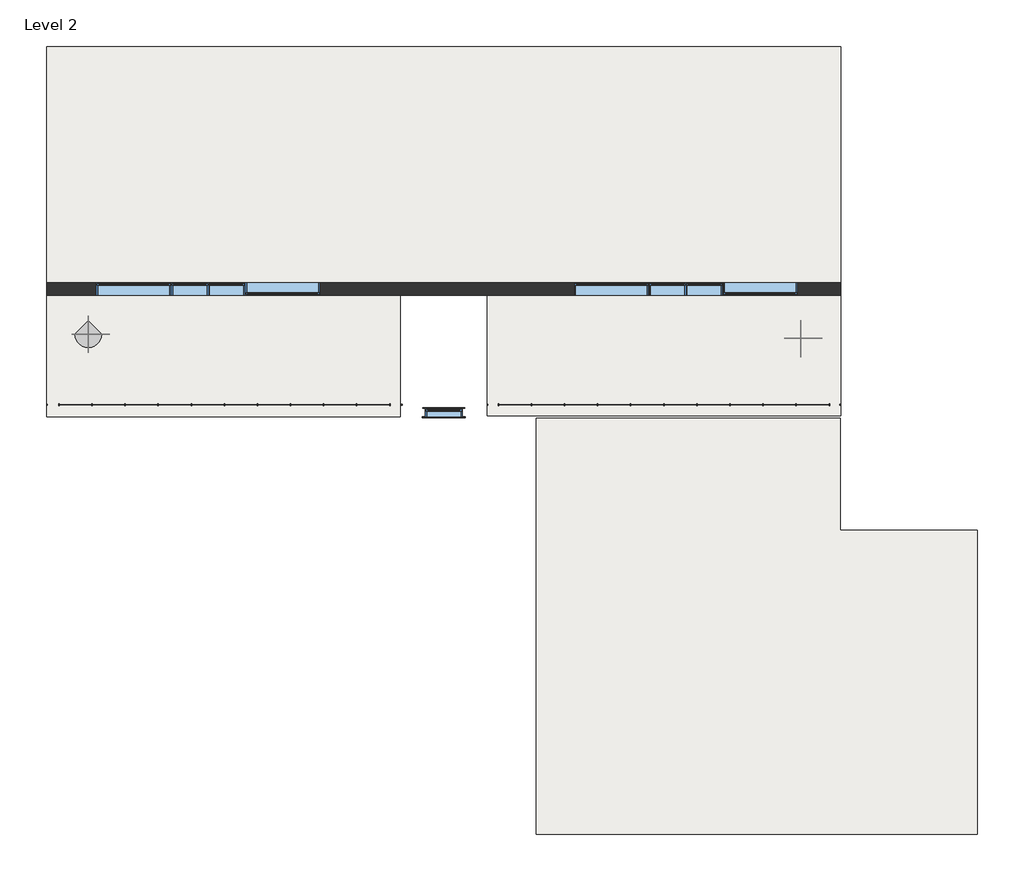
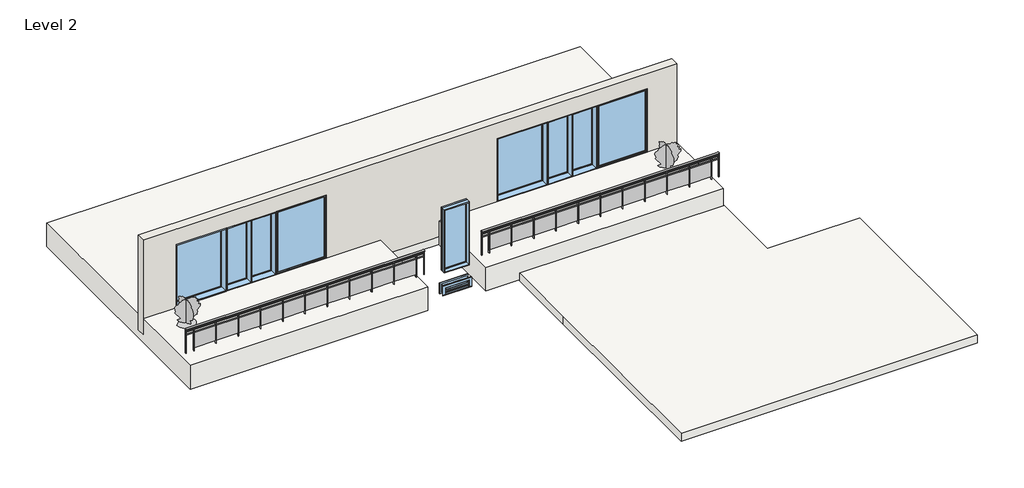
# One storey: 10 windows, 2 geographic elements, 2 railings, 2 slabs, 1 wall.
"""IFC4 building model written with IfcOpenShell, lengths in millimetres."""

from ifc_helpers import new_model, si_unit, point, frame, origin, place, context, project, spatial, polyline, ellipse_curve, trimmed, outline, extrude, faceted_brep, transform, mapped, element, save
from ifc_brep_helpers import plane_surface, extruded_surface, advanced_brep
from components import geographic_element_e27c54a3, window_e4bd14ab, window_a209d960, window_307ff736, window_1de08d8e, window_9610881e

model = new_model("IFC4")

# Units and contexts
model_context = context("Model", 3, world=origin())
ifc_project = project(units=[si_unit("LENGTHUNIT", "METRE", prefix="MILLI")], contexts=[model_context])

# Site, building, storey
site = spatial("IfcSite", under=ifc_project)
building = spatial("IfcBuilding", under=site)
storey = spatial("IfcBuildingStorey", under=building, Name="Level 2", Elevation=3048.0)

# Geographic elements
placement = place(None, origin())
geographic_element_shape = geographic_element_e27c54a3(model_context)
element("IfcGeographicElement", 1, ObjectType="RPC Shrub : Cedar Shrub 3'-0\"", at=placement, inside=storey, context=model_context, shape_type="MappedRepresentation", body=[
    mapped(geographic_element_shape, transform((827.7661524, 4826.2223265, 3657.6), x_axis=(1.0, 0.0, 0.0), y_axis=(0.0, 1.0, 0.0), z_axis=(0.0, 0.0, 1.0))),
])
element("IfcGeographicElement", 2, ObjectType="RPC Shrub : Cedar Shrub 3'-0\"", at=placement, inside=storey, context=model_context, shape_type="MappedRepresentation", body=[
    mapped(geographic_element_shape, transform((-16672.8338476, 4927.8223265, 3740.15), x_axis=(1.0, 0.0, 0.0), y_axis=(0.0, 1.0, 0.0), z_axis=(0.0, 0.0, 1.0))),
])

# Railings
element("IfcRailing", 3, ObjectType="Glass Panel - Bottom Fill", at=placement, inside=storey, context=model_context, shape_type="SolidModel", body=[
    advanced_brep(
    [(-17688.8338476, 3226.0223265, 4876.8), (-17688.8338476, 3149.8223265, 4876.8), (-8966.3603059, 3226.0223265, 4876.8), (-8966.3603059, 3149.8223265, 4876.8)],
    [
        (0, 1, ellipse_curve(frame((-17688.8338476, 3187.9223265, 4876.8), z_axis=(-1.0, 0.0, 0.0), x_axis=(0.0, -1.0, 0.0)), 38.1, 28.575)),
        (1, 0, ellipse_curve(frame((-17688.8338476, 3187.9223265, 4876.8), z_axis=(-1.0, 0.0, 0.0), x_axis=(0.0, -1.0, 0.0)), 38.1, 28.575)),
        (2, 3, ellipse_curve(frame((-8966.3603059, 3187.9223265, 4876.8), z_axis=(1.0, 0.0, 0.0), x_axis=(0.0, -1.0, 0.0)), 38.1, 28.575)),
        (3, 2, ellipse_curve(frame((-8966.3603059, 3187.9223265, 4876.8), z_axis=(1.0, 0.0, 0.0), x_axis=(0.0, -1.0, 0.0)), 38.1, 28.575)),
        (0, 2),
        (3, 1),
    ],
    [
        plane_surface(frame((-17688.8338476, 3187.9223265, 4876.8), z_axis=(-1.0, 0.0, 0.0), x_axis=(0.0, 1.0, 0.0))),
        plane_surface(frame((-8966.3603059, 3187.9223265, 4876.8), z_axis=(1.0, 0.0, 0.0), x_axis=(0.0, 1.0, 0.0))),
        extruded_surface(trimmed(ellipse_curve(frame((-8966.3603059, 3187.9223265, 4876.8), z_axis=(-1.0, 0.0, 0.0), x_axis=(0.0, -1.0, 0.0)), 38.1, 28.575), [point((-8966.3603059, 3226.0223265, 4876.8))], [point((-8966.3603059, 3149.8223265, 4876.8))], True, "CARTESIAN"), (-8722.4735417, 0.0, 0.0), 8722.4735417),
        extruded_surface(trimmed(ellipse_curve(frame((-8966.3603059, 3187.9223265, 4876.8), z_axis=(-1.0, 0.0, 0.0), x_axis=(0.0, -1.0, 0.0)), 38.1, 28.575), [point((-8966.3603059, 3149.8223265, 4876.8))], [point((-8966.3603059, 3226.0223265, 4876.8))], True, "CARTESIAN"), (-8722.4735417, 0.0, 0.0), 8722.4735417),
    ],
    [
        (0, [[1, 2]]),
        (1, [[3, 4]]),
        (2, [[-1, 5, -4, 6]]),
        (3, [[-2, -6, -3, -5]]),
    ],
),
    extrude(outline(polyline([(-17688.8338476, 3175.2223265), (-17688.8338476, 3200.6223265), (-8966.3603059, 3200.6223265), (-8966.3603059, 3175.2223265), (-17688.8338476, 3175.2223265)])), frame((0.0, 0.0, 4762.5), z_axis=(0.0, 0.0, 1.0), x_axis=(1.0, 0.0, 0.0)), (0.0, 0.0, 1.0), 25.4),
    extrude(outline(polyline([(-17688.8338476, 3175.2223265), (-17688.8338476, 3200.6223265), (-8966.3603059, 3200.6223265), (-8966.3603059, 3175.2223265), (-17688.8338476, 3175.2223265)])), frame((0.0, 0.0, 4660.9), z_axis=(0.0, 0.0, 1.0), x_axis=(1.0, 0.0, 0.0)), (0.0, 0.0, 1.0), 25.4),
    extrude(outline(polyline([(-9269.9470767, 3162.5223265), (-9269.9470767, 3213.3223265), (-9257.2470767, 3213.3223265), (-9257.2470767, 3162.5223265), (-9269.9470767, 3162.5223265)])), frame((0.0, 0.0, 3962.4), z_axis=(0.0, 0.0, 1.0), x_axis=(1.0, 0.0, 0.0)), (0.0, 0.0, 1.0), 885.6788223),
    extrude(outline(polyline([(-10076.3970767, 3194.4574835), (-9263.5970767, 3194.4574835), (-9263.5970767, 3188.1074835), (-10076.3970767, 3188.1074835), (-10076.3970767, 3194.4574835)])), frame((0.0, 0.0, 4064.0), z_axis=(0.0, 0.0, 1.0), x_axis=(1.0, 0.0, 0.0)), (0.0, 0.0, 1.0), 596.9),
    extrude(outline(polyline([(-10082.7470767, 3162.5223265), (-10082.7470767, 3213.3223265), (-10070.0470767, 3213.3223265), (-10070.0470767, 3162.5223265), (-10082.7470767, 3162.5223265)])), frame((0.0, 0.0, 3962.4), z_axis=(0.0, 0.0, 1.0), x_axis=(1.0, 0.0, 0.0)), (0.0, 0.0, 1.0), 885.6788223),
    extrude(outline(polyline([(-10889.1970767, 3194.4574835), (-10076.3970767, 3194.4574835), (-10076.3970767, 3188.1074835), (-10889.1970767, 3188.1074835), (-10889.1970767, 3194.4574835)])), frame((0.0, 0.0, 4064.0), z_axis=(0.0, 0.0, 1.0), x_axis=(1.0, 0.0, 0.0)), (0.0, 0.0, 1.0), 596.9),
    extrude(outline(polyline([(-10895.5470767, 3162.5223265), (-10895.5470767, 3213.3223265), (-10882.8470767, 3213.3223265), (-10882.8470767, 3162.5223265), (-10895.5470767, 3162.5223265)])), frame((0.0, 0.0, 3962.4), z_axis=(0.0, 0.0, 1.0), x_axis=(1.0, 0.0, 0.0)), (0.0, 0.0, 1.0), 885.6788223),
    extrude(outline(polyline([(-11701.9970767, 3194.4574835), (-10889.1970767, 3194.4574835), (-10889.1970767, 3188.1074835), (-11701.9970767, 3188.1074835), (-11701.9970767, 3194.4574835)])), frame((0.0, 0.0, 4064.0), z_axis=(0.0, 0.0, 1.0), x_axis=(1.0, 0.0, 0.0)), (0.0, 0.0, 1.0), 596.9),
    extrude(outline(polyline([(-11708.3470767, 3162.5223265), (-11708.3470767, 3213.3223265), (-11695.6470767, 3213.3223265), (-11695.6470767, 3162.5223265), (-11708.3470767, 3162.5223265)])), frame((0.0, 0.0, 3962.4), z_axis=(0.0, 0.0, 1.0), x_axis=(1.0, 0.0, 0.0)), (0.0, 0.0, 1.0), 885.6788223),
    extrude(outline(polyline([(-12514.7970767, 3194.4574835), (-11701.9970767, 3194.4574835), (-11701.9970767, 3188.1074835), (-12514.7970767, 3188.1074835), (-12514.7970767, 3194.4574835)])), frame((0.0, 0.0, 4064.0), z_axis=(0.0, 0.0, 1.0), x_axis=(1.0, 0.0, 0.0)), (0.0, 0.0, 1.0), 596.9),
    extrude(outline(polyline([(-12521.1470767, 3162.5223265), (-12521.1470767, 3213.3223265), (-12508.4470767, 3213.3223265), (-12508.4470767, 3162.5223265), (-12521.1470767, 3162.5223265)])), frame((0.0, 0.0, 3962.4), z_axis=(0.0, 0.0, 1.0), x_axis=(1.0, 0.0, 0.0)), (0.0, 0.0, 1.0), 885.6788223),
    extrude(outline(polyline([(-13327.5970767, 3194.4574835), (-12514.7970767, 3194.4574835), (-12514.7970767, 3188.1074835), (-13327.5970767, 3188.1074835), (-13327.5970767, 3194.4574835)])), frame((0.0, 0.0, 4064.0), z_axis=(0.0, 0.0, 1.0), x_axis=(1.0, 0.0, 0.0)), (0.0, 0.0, 1.0), 596.9),
    extrude(outline(polyline([(-13333.9470767, 3162.5223265), (-13333.9470767, 3213.3223265), (-13321.2470767, 3213.3223265), (-13321.2470767, 3162.5223265), (-13333.9470767, 3162.5223265)])), frame((0.0, 0.0, 3962.4), z_axis=(0.0, 0.0, 1.0), x_axis=(1.0, 0.0, 0.0)), (0.0, 0.0, 1.0), 885.6788223),
    extrude(outline(polyline([(-14140.3970767, 3194.4574835), (-13327.5970767, 3194.4574835), (-13327.5970767, 3188.1074835), (-14140.3970767, 3188.1074835), (-14140.3970767, 3194.4574835)])), frame((0.0, 0.0, 4064.0), z_axis=(0.0, 0.0, 1.0), x_axis=(1.0, 0.0, 0.0)), (0.0, 0.0, 1.0), 596.9),
    extrude(outline(polyline([(-14146.7470767, 3162.5223265), (-14146.7470767, 3213.3223265), (-14134.0470767, 3213.3223265), (-14134.0470767, 3162.5223265), (-14146.7470767, 3162.5223265)])), frame((0.0, 0.0, 3962.4), z_axis=(0.0, 0.0, 1.0), x_axis=(1.0, 0.0, 0.0)), (0.0, 0.0, 1.0), 885.6788223),
    extrude(outline(polyline([(-14953.1970767, 3194.4574835), (-14140.3970767, 3194.4574835), (-14140.3970767, 3188.1074835), (-14953.1970767, 3188.1074835), (-14953.1970767, 3194.4574835)])), frame((0.0, 0.0, 4064.0), z_axis=(0.0, 0.0, 1.0), x_axis=(1.0, 0.0, 0.0)), (0.0, 0.0, 1.0), 596.9),
    extrude(outline(polyline([(-14959.5470767, 3162.5223265), (-14959.5470767, 3213.3223265), (-14946.8470767, 3213.3223265), (-14946.8470767, 3162.5223265), (-14959.5470767, 3162.5223265)])), frame((0.0, 0.0, 3962.4), z_axis=(0.0, 0.0, 1.0), x_axis=(1.0, 0.0, 0.0)), (0.0, 0.0, 1.0), 885.6788223),
    extrude(outline(polyline([(-15765.9970767, 3194.4574835), (-14953.1970767, 3194.4574835), (-14953.1970767, 3188.1074835), (-15765.9970767, 3188.1074835), (-15765.9970767, 3194.4574835)])), frame((0.0, 0.0, 4064.0), z_axis=(0.0, 0.0, 1.0), x_axis=(1.0, 0.0, 0.0)), (0.0, 0.0, 1.0), 596.9),
    extrude(outline(polyline([(-15772.3470767, 3162.5223265), (-15772.3470767, 3213.3223265), (-15759.6470767, 3213.3223265), (-15759.6470767, 3162.5223265), (-15772.3470767, 3162.5223265)])), frame((0.0, 0.0, 3962.4), z_axis=(0.0, 0.0, 1.0), x_axis=(1.0, 0.0, 0.0)), (0.0, 0.0, 1.0), 885.6788223),
    extrude(outline(polyline([(-16578.7970767, 3194.4574835), (-15765.9970767, 3194.4574835), (-15765.9970767, 3188.1074835), (-16578.7970767, 3188.1074835), (-16578.7970767, 3194.4574835)])), frame((0.0, 0.0, 4064.0), z_axis=(0.0, 0.0, 1.0), x_axis=(1.0, 0.0, 0.0)), (0.0, 0.0, 1.0), 596.9),
    extrude(outline(polyline([(-16585.1470767, 3162.5223265), (-16585.1470767, 3213.3223265), (-16572.4470767, 3213.3223265), (-16572.4470767, 3162.5223265), (-16585.1470767, 3162.5223265)])), frame((0.0, 0.0, 3962.4), z_axis=(0.0, 0.0, 1.0), x_axis=(1.0, 0.0, 0.0)), (0.0, 0.0, 1.0), 885.6788223),
    extrude(outline(polyline([(-17391.5970767, 3194.4574835), (-16578.7970767, 3194.4574835), (-16578.7970767, 3188.1074835), (-17391.5970767, 3188.1074835), (-17391.5970767, 3194.4574835)])), frame((0.0, 0.0, 4064.0), z_axis=(0.0, 0.0, 1.0), x_axis=(1.0, 0.0, 0.0)), (0.0, 0.0, 1.0), 596.9),
    extrude(outline(polyline([(-17397.9470767, 3162.5223265), (-17397.9470767, 3213.3223265), (-17385.2470767, 3213.3223265), (-17385.2470767, 3162.5223265), (-17397.9470767, 3162.5223265)])), frame((0.0, 0.0, 3962.4), z_axis=(0.0, 0.0, 1.0), x_axis=(1.0, 0.0, 0.0)), (0.0, 0.0, 1.0), 885.6788223),
    extrude(outline(polyline([(-8979.0603059, 3178.3973265), (-8979.0603059, 3197.4473265), (-8960.0103059, 3197.4473265), (-8960.0103059, 3178.3973265), (-8979.0603059, 3178.3973265)])), frame((0.0, 0.0, 3962.4), z_axis=(0.0, 0.0, 1.0), x_axis=(1.0, 0.0, 0.0)), (0.0, 0.0, 1.0), 885.6788223),
    extrude(outline(polyline([(-17695.1838476, 3178.3973265), (-17695.1838476, 3197.4473265), (-17676.1338476, 3197.4473265), (-17676.1338476, 3178.3973265), (-17695.1838476, 3178.3973265)])), frame((0.0, 0.0, 3962.4), z_axis=(0.0, 0.0, 1.0), x_axis=(1.0, 0.0, 0.0)), (0.0, 0.0, 1.0), 885.6788223),
])
element("IfcRailing", 4, ObjectType="Glass Panel - Bottom Fill", at=placement, inside=storey, context=model_context, shape_type="SolidModel", body=[
    advanced_brep(
    [(-6868.4338476, 3226.0223265, 4876.8), (-6868.4338476, 3149.8223265, 4876.8), (1803.2396941, 3226.0223265, 4876.8), (1803.2396941, 3149.8223265, 4876.8)],
    [
        (0, 1, ellipse_curve(frame((-6868.4338476, 3187.9223265, 4876.8), z_axis=(-1.0, 0.0, 0.0), x_axis=(0.0, -1.0, 0.0)), 38.1, 28.575)),
        (1, 0, ellipse_curve(frame((-6868.4338476, 3187.9223265, 4876.8), z_axis=(-1.0, 0.0, 0.0), x_axis=(0.0, -1.0, 0.0)), 38.1, 28.575)),
        (2, 3, ellipse_curve(frame((1803.2396941, 3187.9223265, 4876.8), z_axis=(1.0, 0.0, 0.0), x_axis=(0.0, -1.0, 0.0)), 38.1, 28.575)),
        (3, 2, ellipse_curve(frame((1803.2396941, 3187.9223265, 4876.8), z_axis=(1.0, 0.0, 0.0), x_axis=(0.0, -1.0, 0.0)), 38.1, 28.575)),
        (0, 2),
        (3, 1),
    ],
    [
        plane_surface(frame((-6868.4338476, 3187.9223265, 4876.8), z_axis=(-1.0, 0.0, 0.0), x_axis=(0.0, 1.0, 0.0))),
        plane_surface(frame((1803.2396941, 3187.9223265, 4876.8), z_axis=(1.0, 0.0, 0.0), x_axis=(0.0, 1.0, 0.0))),
        extruded_surface(trimmed(ellipse_curve(frame((1803.2396941, 3187.9223265, 4876.8), z_axis=(-1.0, 0.0, 0.0), x_axis=(0.0, -1.0, 0.0)), 38.1, 28.575), [point((1803.2396941, 3226.0223265, 4876.8))], [point((1803.2396941, 3149.8223265, 4876.8))], True, "CARTESIAN"), (-8671.6735417, 0.0, 0.0), 8671.6735417),
        extruded_surface(trimmed(ellipse_curve(frame((1803.2396941, 3187.9223265, 4876.8), z_axis=(-1.0, 0.0, 0.0), x_axis=(0.0, -1.0, 0.0)), 38.1, 28.575), [point((1803.2396941, 3149.8223265, 4876.8))], [point((1803.2396941, 3226.0223265, 4876.8))], True, "CARTESIAN"), (-8671.6735417, 0.0, 0.0), 8671.6735417),
    ],
    [
        (0, [[1, 2]]),
        (1, [[3, 4]]),
        (2, [[-1, 5, -4, 6]]),
        (3, [[-2, -6, -3, -5]]),
    ],
),
    extrude(outline(polyline([(-6868.4338476, 3175.2223265), (-6868.4338476, 3200.6223265), (1803.2396941, 3200.6223265), (1803.2396941, 3175.2223265), (-6868.4338476, 3175.2223265)])), frame((0.0, 0.0, 4762.5), z_axis=(0.0, 0.0, 1.0), x_axis=(1.0, 0.0, 0.0)), (0.0, 0.0, 1.0), 25.4),
    extrude(outline(polyline([(-6868.4338476, 3175.2223265), (-6868.4338476, 3200.6223265), (1803.2396941, 3200.6223265), (1803.2396941, 3175.2223265), (-6868.4338476, 3175.2223265)])), frame((0.0, 0.0, 4660.9), z_axis=(0.0, 0.0, 1.0), x_axis=(1.0, 0.0, 0.0)), (0.0, 0.0, 1.0), 25.4),
    extrude(outline(polyline([(1525.0529233, 3162.5223265), (1525.0529233, 3213.3223265), (1537.7529233, 3213.3223265), (1537.7529233, 3162.5223265), (1525.0529233, 3162.5223265)])), frame((0.0, 0.0, 3962.4), z_axis=(0.0, 0.0, 1.0), x_axis=(1.0, 0.0, 0.0)), (0.0, 0.0, 1.0), 885.6788223),
    extrude(outline(polyline([(718.6029233, 3194.4574835), (1531.4029233, 3194.4574835), (1531.4029233, 3188.1074835), (718.6029233, 3188.1074835), (718.6029233, 3194.4574835)])), frame((0.0, 0.0, 4064.0), z_axis=(0.0, 0.0, 1.0), x_axis=(1.0, 0.0, 0.0)), (0.0, 0.0, 1.0), 596.9),
    extrude(outline(polyline([(712.2529233, 3162.5223265), (712.2529233, 3213.3223265), (724.9529233, 3213.3223265), (724.9529233, 3162.5223265), (712.2529233, 3162.5223265)])), frame((0.0, 0.0, 3962.4), z_axis=(0.0, 0.0, 1.0), x_axis=(1.0, 0.0, 0.0)), (0.0, 0.0, 1.0), 885.6788223),
    extrude(outline(polyline([(-94.1970767, 3194.4574835), (718.6029233, 3194.4574835), (718.6029233, 3188.1074835), (-94.1970767, 3188.1074835), (-94.1970767, 3194.4574835)])), frame((0.0, 0.0, 4064.0), z_axis=(0.0, 0.0, 1.0), x_axis=(1.0, 0.0, 0.0)), (0.0, 0.0, 1.0), 596.9),
    extrude(outline(polyline([(-100.5470767, 3162.5223265), (-100.5470767, 3213.3223265), (-87.8470767, 3213.3223265), (-87.8470767, 3162.5223265), (-100.5470767, 3162.5223265)])), frame((0.0, 0.0, 3962.4), z_axis=(0.0, 0.0, 1.0), x_axis=(1.0, 0.0, 0.0)), (0.0, 0.0, 1.0), 885.6788223),
    extrude(outline(polyline([(-906.9970767, 3194.4574835), (-94.1970767, 3194.4574835), (-94.1970767, 3188.1074835), (-906.9970767, 3188.1074835), (-906.9970767, 3194.4574835)])), frame((0.0, 0.0, 4064.0), z_axis=(0.0, 0.0, 1.0), x_axis=(1.0, 0.0, 0.0)), (0.0, 0.0, 1.0), 596.9),
    extrude(outline(polyline([(-913.3470767, 3162.5223265), (-913.3470767, 3213.3223265), (-900.6470767, 3213.3223265), (-900.6470767, 3162.5223265), (-913.3470767, 3162.5223265)])), frame((0.0, 0.0, 3962.4), z_axis=(0.0, 0.0, 1.0), x_axis=(1.0, 0.0, 0.0)), (0.0, 0.0, 1.0), 885.6788223),
    extrude(outline(polyline([(-1719.7970767, 3194.4574835), (-906.9970767, 3194.4574835), (-906.9970767, 3188.1074835), (-1719.7970767, 3188.1074835), (-1719.7970767, 3194.4574835)])), frame((0.0, 0.0, 4064.0), z_axis=(0.0, 0.0, 1.0), x_axis=(1.0, 0.0, 0.0)), (0.0, 0.0, 1.0), 596.9),
    extrude(outline(polyline([(-1726.1470767, 3162.5223265), (-1726.1470767, 3213.3223265), (-1713.4470767, 3213.3223265), (-1713.4470767, 3162.5223265), (-1726.1470767, 3162.5223265)])), frame((0.0, 0.0, 3962.4), z_axis=(0.0, 0.0, 1.0), x_axis=(1.0, 0.0, 0.0)), (0.0, 0.0, 1.0), 885.6788223),
    extrude(outline(polyline([(-2532.5970767, 3194.4574835), (-1719.7970767, 3194.4574835), (-1719.7970767, 3188.1074835), (-2532.5970767, 3188.1074835), (-2532.5970767, 3194.4574835)])), frame((0.0, 0.0, 4064.0), z_axis=(0.0, 0.0, 1.0), x_axis=(1.0, 0.0, 0.0)), (0.0, 0.0, 1.0), 596.9),
    extrude(outline(polyline([(-2538.9470767, 3162.5223265), (-2538.9470767, 3213.3223265), (-2526.2470767, 3213.3223265), (-2526.2470767, 3162.5223265), (-2538.9470767, 3162.5223265)])), frame((0.0, 0.0, 3962.4), z_axis=(0.0, 0.0, 1.0), x_axis=(1.0, 0.0, 0.0)), (0.0, 0.0, 1.0), 885.6788223),
    extrude(outline(polyline([(-3345.3970767, 3194.4574835), (-2532.5970767, 3194.4574835), (-2532.5970767, 3188.1074835), (-3345.3970767, 3188.1074835), (-3345.3970767, 3194.4574835)])), frame((0.0, 0.0, 4064.0), z_axis=(0.0, 0.0, 1.0), x_axis=(1.0, 0.0, 0.0)), (0.0, 0.0, 1.0), 596.9),
    extrude(outline(polyline([(-3351.7470767, 3162.5223265), (-3351.7470767, 3213.3223265), (-3339.0470767, 3213.3223265), (-3339.0470767, 3162.5223265), (-3351.7470767, 3162.5223265)])), frame((0.0, 0.0, 3962.4), z_axis=(0.0, 0.0, 1.0), x_axis=(1.0, 0.0, 0.0)), (0.0, 0.0, 1.0), 885.6788223),
    extrude(outline(polyline([(-4158.1970767, 3194.4574835), (-3345.3970767, 3194.4574835), (-3345.3970767, 3188.1074835), (-4158.1970767, 3188.1074835), (-4158.1970767, 3194.4574835)])), frame((0.0, 0.0, 4064.0), z_axis=(0.0, 0.0, 1.0), x_axis=(1.0, 0.0, 0.0)), (0.0, 0.0, 1.0), 596.9),
    extrude(outline(polyline([(-4164.5470767, 3162.5223265), (-4164.5470767, 3213.3223265), (-4151.8470767, 3213.3223265), (-4151.8470767, 3162.5223265), (-4164.5470767, 3162.5223265)])), frame((0.0, 0.0, 3962.4), z_axis=(0.0, 0.0, 1.0), x_axis=(1.0, 0.0, 0.0)), (0.0, 0.0, 1.0), 885.6788223),
    extrude(outline(polyline([(-4970.9970767, 3194.4574835), (-4158.1970767, 3194.4574835), (-4158.1970767, 3188.1074835), (-4970.9970767, 3188.1074835), (-4970.9970767, 3194.4574835)])), frame((0.0, 0.0, 4064.0), z_axis=(0.0, 0.0, 1.0), x_axis=(1.0, 0.0, 0.0)), (0.0, 0.0, 1.0), 596.9),
    extrude(outline(polyline([(-4977.3470767, 3162.5223265), (-4977.3470767, 3213.3223265), (-4964.6470767, 3213.3223265), (-4964.6470767, 3162.5223265), (-4977.3470767, 3162.5223265)])), frame((0.0, 0.0, 3962.4), z_axis=(0.0, 0.0, 1.0), x_axis=(1.0, 0.0, 0.0)), (0.0, 0.0, 1.0), 885.6788223),
    extrude(outline(polyline([(-5783.7970767, 3194.4574835), (-4970.9970767, 3194.4574835), (-4970.9970767, 3188.1074835), (-5783.7970767, 3188.1074835), (-5783.7970767, 3194.4574835)])), frame((0.0, 0.0, 4064.0), z_axis=(0.0, 0.0, 1.0), x_axis=(1.0, 0.0, 0.0)), (0.0, 0.0, 1.0), 596.9),
    extrude(outline(polyline([(-5790.1470767, 3162.5223265), (-5790.1470767, 3213.3223265), (-5777.4470767, 3213.3223265), (-5777.4470767, 3162.5223265), (-5790.1470767, 3162.5223265)])), frame((0.0, 0.0, 3962.4), z_axis=(0.0, 0.0, 1.0), x_axis=(1.0, 0.0, 0.0)), (0.0, 0.0, 1.0), 885.6788223),
    extrude(outline(polyline([(-6596.5970767, 3194.4574835), (-5783.7970767, 3194.4574835), (-5783.7970767, 3188.1074835), (-6596.5970767, 3188.1074835), (-6596.5970767, 3194.4574835)])), frame((0.0, 0.0, 4064.0), z_axis=(0.0, 0.0, 1.0), x_axis=(1.0, 0.0, 0.0)), (0.0, 0.0, 1.0), 596.9),
    extrude(outline(polyline([(-6602.9470767, 3162.5223265), (-6602.9470767, 3213.3223265), (-6590.2470767, 3213.3223265), (-6590.2470767, 3162.5223265), (-6602.9470767, 3162.5223265)])), frame((0.0, 0.0, 3962.4), z_axis=(0.0, 0.0, 1.0), x_axis=(1.0, 0.0, 0.0)), (0.0, 0.0, 1.0), 885.6788223),
    extrude(outline(polyline([(1790.5396941, 3178.3973265), (1790.5396941, 3197.4473265), (1809.5896941, 3197.4473265), (1809.5896941, 3178.3973265), (1790.5396941, 3178.3973265)])), frame((0.0, 0.0, 3962.4), z_axis=(0.0, 0.0, 1.0), x_axis=(1.0, 0.0, 0.0)), (0.0, 0.0, 1.0), 885.6788223),
    extrude(outline(polyline([(-6874.7838476, 3178.3973265), (-6874.7838476, 3197.4473265), (-6855.7338476, 3197.4473265), (-6855.7338476, 3178.3973265), (-6874.7838476, 3178.3973265)])), frame((0.0, 0.0, 3962.4), z_axis=(0.0, 0.0, 1.0), x_axis=(1.0, 0.0, 0.0)), (0.0, 0.0, 1.0), 885.6788223),
])

# Slabs
element("IfcSlab", 5, ObjectType="Generic - 12\"", at=placement, inside=storey, context=model_context, shape_type="SweptSolid", body=[
    extrude(outline(polyline([(5171.1661524, 110.8416168), (5171.1661524, -7356.7583832), (-5664.3603059, -7356.7583832), (-5664.3603059, 101.8223265), (-5664.3603059, 2854.0416168), (1803.2396941, 2854.0416168), (1803.2396941, 110.8416168), (5171.1661524, 110.8416168)])), frame((0.0, 0.0, 2743.2), z_axis=(0.0, 0.0, 1.0), x_axis=(1.0, 0.0, 0.0)), (0.0, 0.0, 1.0), 304.8),
])
element("IfcSlab", 6, ObjectType="Generic - 3'", at=placement, inside=storey, context=model_context, shape_type="SweptSolid", body=[
    extrude(outline(polyline([(1818.3661524, 11989.0223265), (1818.3661524, 2921.2223265), (-6868.4338476, 2921.2223265), (-6868.4338476, 5893.0223265), (-9002.0338476, 5893.0223265), (-9002.0338476, 2895.8223265), (-17688.8338476, 2895.8223265), (-17688.8338476, 11989.0223265), (1818.3661524, 11989.0223265)])), frame((0.0, 0.0, 2743.2), z_axis=(0.0, 0.0, 1.0), x_axis=(1.0, 0.0, 0.0)), (0.0, 0.0, 1.0), 914.4),
])

# Wall
element("IfcWall", 7, ObjectType="Generic - 12\" black", at=placement, inside=storey, context=model_context, shape_type="Brep", body=[
    faceted_brep([(-17688.8338476, 5880.3223265, 3048.0), (-9002.0338476, 5880.3223265, 3048.0), (-8697.2338476, 5880.3223265, 3048.0), (-7173.2338476, 5880.3223265, 3048.0), (-6868.4338476, 5880.3223265, 3048.0), (1818.3661524, 5880.3223265, 3048.0), (1818.3661524, 5880.3223265, 6705.6), (-17688.8338476, 5880.3223265, 6705.6), (-14640.8338476, 5880.3223265, 6096.0), (-14640.8338476, 5880.3223265, 3657.6), (-16469.6338476, 5880.3223265, 3657.6), (-16469.6338476, 5880.3223265, 6096.0), (-14631.3088476, 5880.3223265, 3651.883689), (-14631.3088476, 5880.3223265, 6090.283689), (-12821.5588476, 5880.3223265, 6090.283689), (-12821.5588476, 5880.3223265, 3651.883689), (-10983.2338476, 5880.3223265, 6096.0), (-10983.2338476, 5880.3223265, 3657.6), (-12812.0338476, 5880.3223265, 3657.6), (-12812.0338476, 5880.3223265, 6096.0), (751.5661524, 5880.3223265, 6096.0), (751.5661524, 5880.3223265, 3657.6), (-1077.2338476, 5880.3223265, 3657.6), (-1077.2338476, 5880.3223265, 6096.0), (-2896.5088476, 5880.3223265, 6090.283689), (-1086.7588476, 5880.3223265, 6090.283689), (-1086.7588476, 5880.3223265, 3651.883689), (-2896.5088476, 5880.3223265, 3651.883689), (-2906.0338476, 5880.3223265, 6096.0), (-2906.0338476, 5880.3223265, 3657.6), (-4734.8338476, 5880.3223265, 3657.6), (-4734.8338476, 5880.3223265, 6096.0), (1818.3661524, 6185.1223265, 3048.0), (-17688.8338476, 6185.1223265, 3048.0), (-17688.8338476, 6185.1223265, 6705.6), (1818.3661524, 6185.1223265, 6705.6), (-14640.8338476, 6185.1223265, 6096.0), (-16469.6338476, 6185.1223265, 6096.0), (-16469.6338476, 6185.1223265, 3657.6), (-14640.8338476, 6185.1223265, 3657.6), (-14631.3088476, 6185.1223265, 6090.283689), (-14631.3088476, 6185.1223265, 3651.883689), (-12821.5588476, 6185.1223265, 3651.883689), (-12821.5588476, 6185.1223265, 6090.283689), (-10983.2338476, 6185.1223265, 6096.0), (-12812.0338476, 6185.1223265, 6096.0), (-12812.0338476, 6185.1223265, 3657.6), (-10983.2338476, 6185.1223265, 3657.6), (751.5661524, 6185.1223265, 6096.0), (-1077.2338476, 6185.1223265, 6096.0), (-1077.2338476, 6185.1223265, 3657.6), (751.5661524, 6185.1223265, 3657.6), (-2896.5088476, 6185.1223265, 3651.883689), (-1086.7588476, 6185.1223265, 3651.883689), (-1086.7588476, 6185.1223265, 6090.283689), (-2896.5088476, 6185.1223265, 6090.283689), (-2906.0338476, 6185.1223265, 6096.0), (-4734.8338476, 6185.1223265, 6096.0), (-4734.8338476, 6185.1223265, 3657.6), (-2906.0338476, 6185.1223265, 3657.6)], [[[0, 1, 2, 3, 4, 5, 6, 7], [8, 9, 10, 11], [12, 13, 14, 15], [16, 17, 18, 19], [20, 21, 22, 23], [24, 25, 26, 27], [28, 29, 30, 31]], [[32, 33, 34, 35], [36, 37, 38, 39], [40, 41, 42, 43], [44, 45, 46, 47], [48, 49, 50, 51], [52, 53, 54, 55], [56, 57, 58, 59]], [[5, 4, 3, 2, 1, 0, 33, 32]], [[7, 6, 35, 34]], [[0, 7, 34, 33]], [[6, 5, 32, 35]], [[9, 8, 36, 39]], [[10, 9, 39, 38]], [[11, 10, 38, 37]], [[8, 11, 37, 36]], [[41, 12, 15, 42]], [[13, 12, 41, 40]], [[13, 40, 43, 14]], [[14, 43, 42, 15]], [[17, 16, 44, 47]], [[18, 17, 47, 46]], [[19, 18, 46, 45]], [[16, 19, 45, 44]], [[21, 20, 48, 51]], [[22, 21, 51, 50]], [[23, 22, 50, 49]], [[20, 23, 49, 48]], [[26, 25, 54, 53]], [[26, 53, 52, 27]], [[54, 25, 24, 55]], [[27, 52, 55, 24]], [[29, 28, 56, 59]], [[30, 29, 59, 58]], [[31, 30, 58, 57]], [[28, 31, 57, 56]]]),
])

# Windows
window_shape = window_e4bd14ab(model_context)
element("IfcWindow", 8, ObjectType="Double Hung with Trim : 36\" x 12\"", at=placement, inside=storey, context=model_context, shape_type="MappedRepresentation", body=[
    mapped(window_shape, transform((-7935.2338476, 2997.4223265, 2212.4251543), x_axis=(-1.0, 0.0, 0.0), y_axis=(0.0, -1.0, 0.0), z_axis=(0.0, 0.0, 1.0))),
])
window_2_shape = window_a209d960(model_context)
element("IfcWindow", 9, ObjectType="Fixed : 36\" x 96\"", at=placement, inside=storey, context=model_context, shape_type="MappedRepresentation", body=[
    mapped(window_2_shape, transform((-14136.0088476, 6032.7223265, 3347.083689), x_axis=(1.0, 0.0, 0.0), y_axis=(0.0, 1.0, 0.0), z_axis=(0.0, 0.0, 1.0))),
])
element("IfcWindow", 10, ObjectType="Fixed : 36\" x 96\"", at=placement, inside=storey, context=model_context, shape_type="MappedRepresentation", body=[
    mapped(window_2_shape, transform((-13240.6588476, 6032.7223265, 3347.083689), x_axis=(1.0, 0.0, 0.0), y_axis=(0.0, 1.0, 0.0), z_axis=(0.0, 0.0, 1.0))),
])
element("IfcWindow", 11, ObjectType="Fixed : 36\" x 96\"", at=placement, inside=storey, context=model_context, shape_type="MappedRepresentation", body=[
    mapped(window_2_shape, transform((-2401.2088476, 6032.7223265, 3347.083689), x_axis=(1.0, 0.0, 0.0), y_axis=(0.0, 1.0, 0.0), z_axis=(0.0, 0.0, 1.0))),
])
element("IfcWindow", 12, ObjectType="Fixed : 36\" x 96\"", at=placement, inside=storey, context=model_context, shape_type="MappedRepresentation", body=[
    mapped(window_2_shape, transform((-1505.8588476, 6032.7223265, 3347.083689), x_axis=(1.0, 0.0, 0.0), y_axis=(0.0, 1.0, 0.0), z_axis=(0.0, 0.0, 1.0))),
])
window_3_shape = window_307ff736(model_context)
element("IfcWindow", 13, ObjectType="Fixed : 36\" x 96\"", at=placement, inside=storey, context=model_context, shape_type="MappedRepresentation", body=[
    mapped(window_3_shape, transform((-7897.1338476, 2997.4223265, 3676.4691739), x_axis=(1.0, 0.0, 0.0), y_axis=(0.0, 1.0, 0.0), z_axis=(0.0, 0.0, 1.0))),
])
window_4_shape = window_1de08d8e(model_context)
element("IfcWindow", 14, ObjectType="Fixed : 72\" x 96\"", at=placement, inside=storey, context=model_context, shape_type="MappedRepresentation", body=[
    mapped(window_4_shape, transform((-15517.1338476, 6032.7223265, 3352.8), x_axis=(1.0, 0.0, 0.0), y_axis=(0.0, 1.0, 0.0), z_axis=(0.0, 0.0, 1.0))),
])
element("IfcWindow", 15, ObjectType="Fixed : 72\" x 96\"", at=placement, inside=storey, context=model_context, shape_type="MappedRepresentation", body=[
    mapped(window_4_shape, transform((-3782.3338476, 6032.7223265, 3352.8), x_axis=(1.0, 0.0, 0.0), y_axis=(0.0, 1.0, 0.0), z_axis=(0.0, 0.0, 1.0))),
])
window_5_shape = window_9610881e(model_context)
element("IfcWindow", 16, ObjectType="Fixed : 72\" x 96\"", at=placement, inside=storey, context=model_context, shape_type="MappedRepresentation", body=[
    mapped(window_5_shape, transform((-11859.5338476, 6032.7223265, 3352.8), x_axis=(1.0, 0.0, 0.0), y_axis=(0.0, 1.0, 0.0), z_axis=(0.0, 0.0, 1.0))),
])
element("IfcWindow", 17, ObjectType="Fixed : 72\" x 96\"", at=placement, inside=storey, context=model_context, shape_type="MappedRepresentation", body=[
    mapped(window_5_shape, transform((-124.7338476, 6032.7223265, 3352.8), x_axis=(1.0, 0.0, 0.0), y_axis=(0.0, 1.0, 0.0), z_axis=(0.0, 0.0, 1.0))),
])

save(model, "model.ifc")

# Revit data of these elements
# Type "RPC Shrub : Cedar Shrub 3'-0\""
#   Type Comments = "Cedar Shrub"
#   built-in parameter 1005198 = "{2, 15},{39, RPC-16-FUMD-ULXX-U7X6-J000-ST1L-LVER-AU},{1, 0},{1, 0},{2, 13},{1, 8},{5, Color},{1, 0},{1, 0},{3, 0.8},{3, 0.8},{3, 0.8},{1, 8},{7, BBoxMin},{1, 0},{1, 0},{1, 0},{1, 0},{1, 0},{1, 8},{7, BBoxMax},{1, 0},{1, 0},{1, 0},{1, 0},{1, 0},{2, 11},{9, RPCTypeId},{1, 0},{1, 0},{39, RPC-16-FUMD-ULXX-U7X6-J000-ST1L-LVER-AU},{1, 6},{14, RPCPlantHeight},{1, 0},{1, 0},{1, 3},{2, 11},{7, keyword},{1, 0},{1, 0},{35, :RPCs:Shrubs [General]:Geometry:RPC},{2, 11},{8, category},{1, 0},{1, 0},{16, Shrubs [General]},{2, 11},{12, LocalizedUID},{1, 0},{1, 0},{11, Cedar Shrub},{2, 14},{6, Height},{1, 0},{1, 0},{1, 3},{1, 2},{16, Cast Reflections},{1, 0},{1, 0},{1, 0},{1, 2},{12, Cast Shadows},{1, 0},{1, 0},{1, 1},{1, 2},{9, Lock View},{1, 0},{1, 0},{1, 0},{1, 4},{5, ViewC},{1, 0},{1, 0},{1, 0},{21, assetlibrary_base.fbx},{1, 5},"
#   built-in parameter 1005195 = "RPC-16-FUMD-ULXX-U7X6-J000-ST1L-LVER-AU"
#   Assembly Code = "G2050500"
#   Height = 3' - 0"
#   Default Elevation = 0
# Type "Glass Panel - Bottom Fill"
#   Assembly Code = "C2010400"
#   built-in parameter 1008612 = 0.0416667 (stored number, unit not read)
#   built-in parameter 1008611 = 0.0416667 (stored number, unit not read)
#   built-in parameter 1008609 = 0.333333 (stored number, unit not read)
#   built-in parameter 1008604 = 0.166667 (stored number, unit not read)
#   built-in parameter 1008603 = 0.166667 (stored number, unit not read)
#   Railing Height = 3' - 0"
#   built-in parameter 1008630 = 2
#   built-in parameter 1008610 = 2
#   built-in parameter 1008618 = Baluster - Square : 3/4"
# Type "Generic - 12\""
#   Assembly Code = "B1010"
#   Function = 0
#   Layers, outside or top first: 1' - 0" "Concrete Masonry Units" (function 1)
# Type "Generic - 3'"
#   Assembly Code = "B1010"
#   Function = 0
#   Layers, outside or top first: 3' - 0" "Concrete Masonry Units" (function 1)
# Type "Generic - 12\" black"
#   Assembly Code = "B2010"
#   Layers, outside or top first: 1' - 0" "Parking Stripe" (function 1)
# Type "Double Hung with Trim : 36\" x 12\""
#   Type Mark = "21"
#   Construction Type Id = "GSP4R"
#   Assembly Code = "B2020100"
#   Analytic Construction = "1/8 in Pilkington single glazing"
#   Visual Light Transmittance = 0.9
#   Solar Heat Gain Coefficient = 0.78
#   Heat Transfer Coefficient (U) = 0.6496 BTU/(h·ft²·°F)
#   Height = 1' - 0"
#   Default Sill Height = 3' - 0"
#   Trim Projection - Ext. = 0' - 0 1/2"
#   Trim Projection - Int. = 0' - 0 3/4"
#   Trim Width - Exterior = 0' - 3 1/2"
#   Trim Width - Interior = 0' - 3 1/2"
#   Width = 3' - 0"
#   Window Inset = 0' - 0 3/4"
#   Define Thermal Properties by = 1
#   Glass Pane Material = Glass
#   Sash Material = Iron, Ductile
#   Trim Exterior Material = Iron, Ductile
#   Trim Interior Material = Iron, Ductile
#   Wall Closure = (empty or 0)
# Type "Fixed : 36\" x 96\""
#   Type Mark = "9"
#   Construction Type Id = "GSP4R"
#   Assembly Code = "B2020100"
#   Analytic Construction = "1/8 in Pilkington single glazing"
#   Visual Light Transmittance = 0.9
#   Solar Heat Gain Coefficient = 0.78
#   Heat Transfer Coefficient (U) = 0.6496 BTU/(h·ft²·°F)
#   Height = 8' - 0"
#   Default Sill Height = 1' - 0"
#   Width = 3' - 0"
#   Window Inset = 0' - 0 3/4"
#   Define Thermal Properties by = 1
#   Glass Pane Material = Glass
#   Sash Material = Iron, Ductile
#   Wall Closure = (empty or 0)
# Type "Fixed : 72\" x 96\""
#   Type Mark = "11"
#   Construction Type Id = "GSP4R"
#   Assembly Code = "B2020100"
#   Analytic Construction = "1/8 in Pilkington single glazing"
#   Visual Light Transmittance = 0.9
#   Solar Heat Gain Coefficient = 0.78
#   Heat Transfer Coefficient (U) = 0.6496 BTU/(h·ft²·°F)
#   Height = 8' - 0"
#   Default Sill Height = 1' - 0"
#   Width = 6' - 0"
#   Window Inset = 0' - 0 3/4"
#   Define Thermal Properties by = 1
#   Glass Pane Material = Glass
#   Sash Material = Iron, Ductile
#   Wall Closure = (empty or 0)
# Elements 1, 2 (IfcGeographicElement, "RPC Shrub : Cedar Shrub 3'-0\"")
#   Phase Created = New Construction
# Elements 3, 4 (IfcRailing, "Glass Panel - Bottom Fill")
#   built-in parameter 1008621 = 3 (stored number, unit not read)
#   Phase Created = New Construction
#   Materials on its faces: "Glass"
# Element 5 (IfcSlab, "Generic - 12\"")
#   built-in parameter 1001955 = 1.5708 (stored number, unit not read)
#   Height Offset From Level = 0' - 0"
#   Phase Created = New Construction
#   Materials on its faces: "Concrete Masonry Units"
# Element 6 (IfcSlab, "Generic - 3'")
#   Height Offset From Level = 2' - 0"
#   Phase Created = New Construction
#   Materials on its faces: "Concrete Masonry Units"
# Element 7 (IfcWall, "Generic - 12\" black")
#   Top Offset = 0' - 0"
#   Base Offset = 0' - 0"
#   Unconnected Height = 12' - 0"
#   wall height = 12' - 0"
#   Phase Created = New Construction
#   Base Constraint = Level 2
#   Materials on its faces: "Parking Stripe"
# Element 8 (IfcWindow, "Double Hung with Trim : 36\" x 12\"")
#   Mark = "27"
#   Phase Created = New Construction
#   Materials on its faces: "Iron, Ductile", "Glass"
# Element 9 (IfcWindow, "Fixed : 36\" x 96\"")
#   Mark = "9"
#   Phase Created = New Construction
#   Materials on its faces: "Iron, Ductile", "Glass"
# Element 10 (IfcWindow, "Fixed : 36\" x 96\"")
#   Mark = "10"
#   Phase Created = New Construction
#   Materials on its faces: "Iron, Ductile", "Glass"
# Element 11 (IfcWindow, "Fixed : 36\" x 96\"")
#   Mark = "13"
#   Phase Created = New Construction
#   Materials on its faces: "Iron, Ductile", "Glass"
# Element 12 (IfcWindow, "Fixed : 36\" x 96\"")
#   Mark = "14"
#   Phase Created = New Construction
#   Materials on its faces: "Iron, Ductile", "Glass"
# Element 13 (IfcWindow, "Fixed : 36\" x 96\"")
#   Mark = "25"
#   Phase Created = New Construction
#   Materials on its faces: "Iron, Ductile", "Glass"
# Element 14 (IfcWindow, "Fixed : 72\" x 96\"")
#   Mark = "8"
#   Phase Created = New Construction
#   Materials on its faces: "Iron, Ductile", "Glass"
# Element 15 (IfcWindow, "Fixed : 72\" x 96\"")
#   Mark = "12"
#   Phase Created = New Construction
#   Materials on its faces: "Iron, Ductile", "Glass"
# Element 16 (IfcWindow, "Fixed : 72\" x 96\"")
#   Mark = "11"
#   Phase Created = New Construction
#   Materials on its faces: "Iron, Ductile", "Glass"
# Element 17 (IfcWindow, "Fixed : 72\" x 96\"")
#   Mark = "15"
#   Phase Created = New Construction
#   Materials on its faces: "Iron, Ductile", "Glass"
# Materials
#   "Concrete Masonry Units": class "Masonry", colour RGB 227 227 227, transparency 0, Description = "Concrete masonry units", Cost = 0
#   "Parking Stripe": class "Paint", colour RGB 250 250 91, transparency 0, Cost = 0
#   "Glass": class "Glass", colour RGB 0 128 192, transparency 0.75, Description = "Soda Lime Glass", Cost = 0
#   "Iron, Ductile": class "Metal", colour RGB 0 0 0, transparency 0, Description = "Ductile cast iron", Cost = 0
